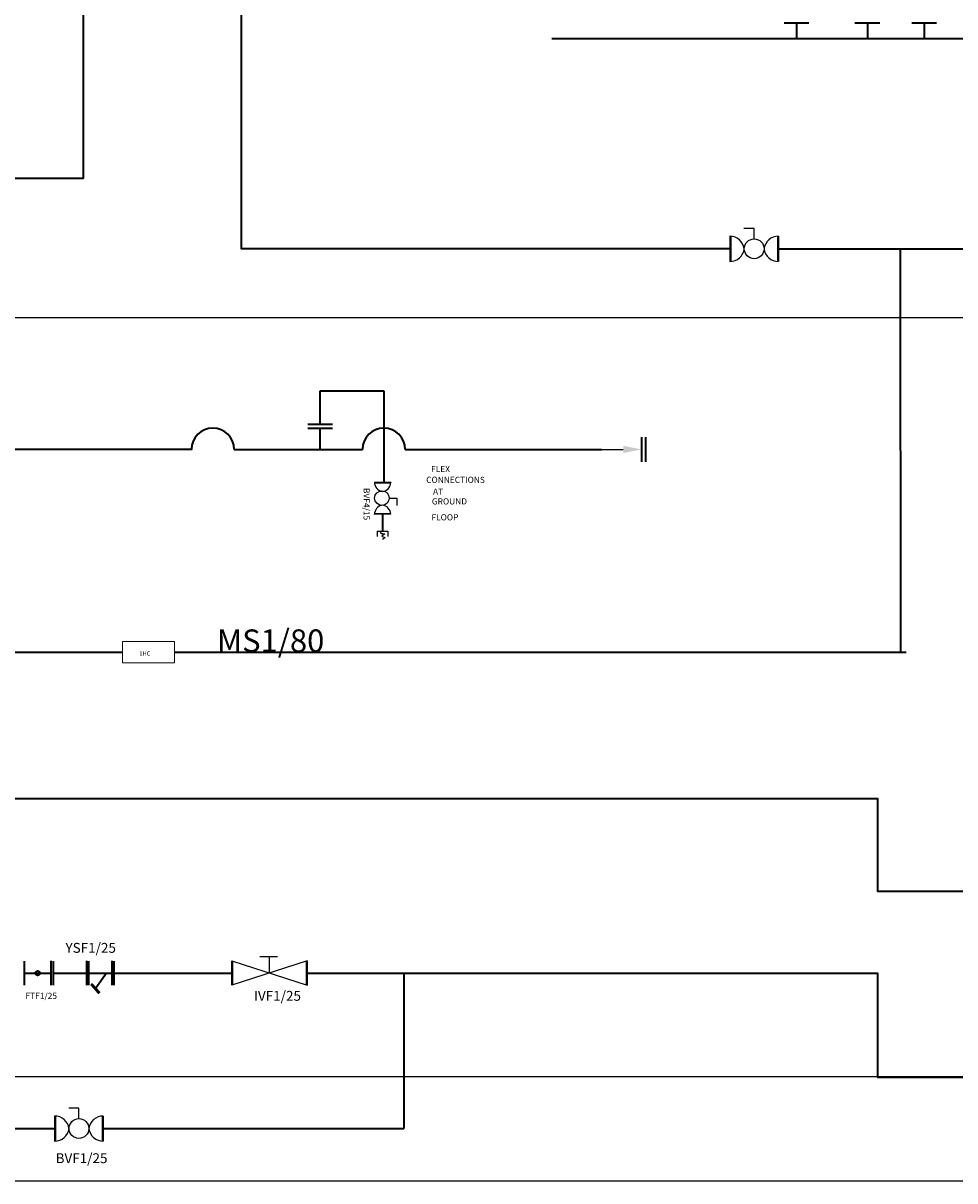
# Model space of a CAD drawing. Units: millimetres. Extents: x 353872 to 441597, y 126154 to 187356.
# Tile 6 of 28: x 381210 to 390443, y 137813 to 149281. Entities that reach past the tile are written whole.
import ezdxf

# ---------------------------------------------------------------- set-up
doc = ezdxf.new("R2010")
doc.units = ezdxf.units.MM
doc.linetypes.add('ACAD_ISO02W100', pattern=[15, 12, -3])
for name, color, linetype, lineweight in [('A-ANNO-DIMS', 2, 'Continuous', 18), ('P-ANNO-TEXT', 7, 'Continuous', 25), ('P-BNDY', 4, 'ACAD_ISO02W100', 25), ('P-INST', 6, 'Continuous', 25), ('P-INST-SIGN', 4, 'Continuous', 18), ('P-PIPE', 3, 'Continuous', 35), ('P-PIPE-FITT', 6, 'Continuous', 25), ('P-VALV', 2, 'Continuous', 25)]:
    doc.layers.add(name, color=color, linetype=linetype, lineweight=lineweight)
doc.layers.add('AC-UINT', color=2, linetype='Continuous')
doc.styles.get("Standard").update_dxf_attribs({"font": 'arial.ttf'})
doc.dimstyles.get("Standard").update_dxf_attribs({"dimtxt": 0.18, "dimasz": 0.18, "dimexe": 0.18, "dimexo": 0.0625, "dimgap": 0.09, "dimtad": 0, "dimtih": 1, "dimtoh": 1, "dimdec": 4, "dimzin": 0, "dimdsep": 46, "dimtxsty": 'Standard', "dimcen": 0.09, "dimadec": 0, "dimazin": 0, "dimtfac": 1, "dimtdec": 4, "dimtofl": 0, "dimtmove": 0, "dimatfit": 3, "dimfxl": 1, "dimtolj": 1, "dimtzin": 0, "dimarcsym": 0})

# ---------------------------------------------------------------- blocks, each defined once
blk = doc.blocks.new('DFSG')
at = {"layer": 'AC-UINT', "ltscale": 3}
blk.add_line((94.324, -27.16), (94.091, -27.16), dxfattribs=at)
blk.add_solid([(94.091, -27.121), (94.091, -27.199), (93.897, -27.16)], dxfattribs=at)
blk = doc.blocks.new('VALVE-A')
for points in [[(0, 9), (249, 9)], [(0, 6), (249, 6)], [(0, 3), (0, 0), (249, 0), (249, 4)], [(0, 3), (0, 3), (246, 3), (249, 3)]]:
    blk.add_lwpolyline(points)
for centre, radius, start, end in [((143, 1), 143, 97.3612, 180.5798), ((107, 2), 142, 359.2193, 82.8397)]:
    blk.add_arc(centre, radius, start, end)
blk = doc.blocks.new('VALVE-D-INDICATOR')
for points in [[(330, 249), (330, 0)], [(333, 249), (333, 0)], [(336, 249), (339, 249), (339, 0), (335, 0)], [(336, 249), (336, 246), (336, 3), (336, 0)]]:
    blk.add_lwpolyline(points)
blk.add_circle((98, 125), 98)
for centre, radius, start, end in [((338, 106), 143, 89.4202, 172.6388), ((337, 142), 142, 187.1603, 270.7807)]:
    blk.add_arc(centre, radius, start, end)
blk = doc.blocks.new('VALVE-K')
for points in [[(0, 91), (0, 93), (162, 93), (162, 90)], [(0, 91), (2, 91), (160, 91), (162, 91)], [(0, 89), (162, 89)], [(0, 87), (161, 87)]]:
    blk.add_lwpolyline(points)
for centre, radius, start, end in [((93, 92), 92.6, 179.4202, 262.6388), ((69, 92), 92.3, 277.1603, 0.7807)]:
    blk.add_arc(centre, radius, start, end)
blk = doc.blocks.new('INST-ELEMENT')
blk.add_lwpolyline([(145, 74), (220, 74), (220, 0)])
blk.add_circle((72, 74), 72.3)
blk = doc.blocks.new('*D27')
at = {"layer": 'A-ANNO-DIMS', "color": 0, "lineweight": -2, "transparency": 16777216}
for p, q in [((366977, 138848), (440591, 138848)), ((440591, 138848), (440591, 138331)), ((440591, 137813), (440591, 138330)), ((366977, 137813), (440591, 137813))]:
    blk.add_line(p, q, dxfattribs=at)
at = {"layer": 'A-ANNO-DIMS', "color": 0, "transparency": 16777216}
for points in [[(440591, 138848), (440591, 138848), (440591, 138848)], [(440591, 137813), (440591, 137813), (440591, 137813)]]:
    blk.add_solid(points, dxfattribs=at)
at = {"layer": 'Defpoints', "color": 0, "transparency": 16777216}
for p in [(366977, 138848), (366977, 137813), (440591, 137813)]:
    blk.add_point(p, dxfattribs=at)
at = {"layer": 'A-ANNO-DIMS', "color": 0, "transparency": 16777216, "insert": (440591, 138330), "char_height": 0.18, "attachment_point": 5}
blk.add_mtext('\\A1;1035.2', dxfattribs=at)

msp = doc.modelspace()

# ---------------------------------------------------------------- linework, layer by layer
at = {"layer": 'P-BNDY'}
msp.add_line((360736.55, 146365.61), (391507.08, 146365.61), dxfattribs=at)
at = {"layer": 'P-INST-SIGN'}
msp.add_lwpolyline([(382194.24, 143154.87), (382709.57, 143154.87), (382709.57, 142945.91), (382194.24, 142945.91)], close=True, dxfattribs=at)
at = {"layer": 'P-PIPE'}
for p, q in [((388996.7, 149280.57), (388751.94, 149280.57)), ((388874.32, 149280.57), (388874.32, 149129.17)), ((389698.22, 149280.57), (389453.46, 149280.57)), ((389575.84, 149280.57), (389575.84, 149129.17)), ((390262.67, 149280.57), (390017.91, 149280.57)), ((390140.29, 149280.57), (390140.29, 149129.17)), ((386450.69, 149129.17), (407087.67, 149129.17)), ((388692.41, 147045.54), (391112.65, 147045.74)), ((389902.53, 147045.64), (389902.86, 143050.39)), ((384154.35, 145309.55), (384154.35, 145637.47)), ((384154.35, 145637.47), (384783.69, 145637.47)), ((384783.69, 145637.47), (384783.69, 144732.81)), ((384031.97, 145309.55), (384276.73, 145309.55)), ((384031.97, 145270.39), (384276.73, 145270.39)), ((384154.35, 145058.64), (384154.35, 145270.39)), ((387336.62, 145179.44), (387336.62, 144934.68)), ((387375.77, 145179.44), (387375.77, 144934.68)), ((383301.45, 145058.64), (384571.94, 145058.64)), ((384995.44, 145058.64), (386942.19, 145058.64)), ((384771.93, 144414.6), (384771.93, 144247.55)), ((382709.57, 143050.39), (389961.77, 143050.39)), ((381219.87, 139989.74), (381219.87, 139751.19)), ((381485.14, 139991.02), (381485.14, 139752.47)), ((381505.55, 139989.74), (381505.55, 139751.19)), ((381838.28, 139991.02), (381838.28, 139752.47)), ((381858.69, 139989.74), (381858.69, 139751.19)), ((382088.51, 139991.02), (382088.51, 139752.47)), ((382108.93, 139989.74), (382108.93, 139751.19)), ((381219.87, 139870.46), (381485.14, 139870.46)), ((381505.55, 139870.46), (381838.28, 139870.46)), ((381858.69, 139870.46), (382088.51, 139870.46)), ((382035.97, 139870.46), (381929.73, 139721.6)), ((382108.93, 139870.46), (383279.44, 139870.46)), ((384981.21, 139870.46), (384981.21, 138330.46)), ((366976.76, 138330.45), (381521.27, 138330.45)), ((382003.25, 138330.46), (384981.21, 138330.46))]:
    msp.add_line(p, q, dxfattribs=at)
for points in [[(366976.76, 171744.89), (381803.29, 171744.89), (381803.29, 150820.94), (381803.29, 147742.48), (377889.79, 147742.48)], [(376740.39, 146769.18), (376740.39, 143050.39), (379096.81, 143050.39), (382194.24, 143050.39)], [(380161.54, 141602.11), (389676.87, 141602.11), (389676.87, 140682.39), (392361.87, 140682.39), (392361.87, 141110.07)], [(384023.46, 139870.46), (389676.87, 139870.46), (389676.87, 138839.25), (395834.15, 138839.25), (395834.15, 140770.36)]]:
    msp.add_lwpolyline(points, dxfattribs=at)
for points in [[(388213.21, 147045.52), (383375.2, 147045.17), (383375.2, 147045.17), (383375.2, 149602.24), (383375.2, 167832.6), (382147.59, 167832.6, 1), (381458.98, 167832.6), (380124.81, 167832.6, 1), (379436.2, 167832.6), (368453.37, 167832.6)], [(383301.45, 145058.64, 1), (382877.96, 145058.64), (377035.77, 145058.64, 1), (376445.02, 145058.64), (372504.41, 145058.64, 1), (371913.66, 145058.64), (366976.76, 145058.64)]]:
    msp.add_lwpolyline(points, format="xyb", dxfattribs=at)
msp.add_lwpolyline([(381884.53, 139753.44), (381894.08, 139761.89), (381965.38, 139681.3), (381955.83, 139672.85)], close=True, dxfattribs=at)
msp.add_circle((381353.34, 139870.46), 22.57, dxfattribs=at)
msp.add_arc((384783.69, 145058.64), 211.75, 0, 180, dxfattribs=at)
at = {"layer": 'P-VALV'}
for p, q in [((383555.44, 140034.39), (383731.66, 140034.39)), ((383651.45, 139870.46), (383651.45, 140034.39)), ((383279.44, 139991.02), (384023.46, 139749.91)), ((384023.46, 139991.02), (383279.44, 139749.91))]:
    msp.add_line(p, q, dxfattribs=at)
for points in [[(388454.2, 147143.89), (388454.2, 147246.54), (388353.42, 147246.54)], [(384720.39, 144195.79), (384720.39, 144247.55), (384823.46, 144247.55), (384823.46, 144195.79)], [(383279.44, 139749.91), (383279.44, 139991.02)], [(383287.34, 139752.47), (383287.34, 139988.45)], [(384015.55, 139988.45), (384015.55, 139752.47)], [(384023.46, 139991.02), (384023.46, 139749.91)], [(381762.26, 138428.82), (381762.26, 138531.46), (381661.48, 138531.46)]]:
    msp.add_lwpolyline(points, dxfattribs=at)
msp.add_open_spline([(384770.05, 144247.55), (384758.68, 144240.53), (384728.6, 144221.95), (384828.65, 144229.34), (384735.73, 144194.17), (384810.98, 144191.29), (384784.82, 144174.67), (384772.32, 144166.73)], degree=3, knots=[0, 0, 0, 0, 27.05142883, 71.59411322, 109.19990694, 141.17080136, 170.38673835, 170.38673835, 170.38673835, 170.38673835], dxfattribs=at)

# ---------------------------------------------------------------- block references
at = {"layer": 'P-INST'}
msp.add_blockref('INST-ELEMENT', (384692.53, 144501.83), dxfattribs=at)
at = {"layer": 'P-PIPE-FITT', "xscale": 923.3484342094463, "yscale": 923.3484342094463, "zscale": 923.3484342094463, "rotation": 179.9589088552121}
msp.add_blockref('DFSG', (474017.82, 119917.94), dxfattribs=at)
at = {"layer": 'P-VALV'}
for name, p, rotation in [('VALVE-A', (388213.21, 147169.91), 269.9999999999359), ('VALVE-K', (384691.22, 144641.64), 0.0028725521061233), ('VALVE-K', (384850.84, 144509.52), 181.3047895544739), ('VALVE-A', (381521.27, 138454.83), 269.9999999998651)]:
    msp.add_blockref(name, p, dxfattribs=dict(at, rotation=rotation))
for p in [(388356.18, 146921.16), (381664.23, 138206.08)]:
    msp.add_blockref('VALVE-D-INDICATOR', p, dxfattribs=at)

# ---------------------------------------------------------------- texts
at = {"layer": 'P-ANNO-TEXT'}
for s, height, p in [('FLEX', 60.86, (385252.41, 144833.81)), ('CONNECTIONS', 60.86, (385203.8, 144726.97)), ('AT', 60.86, (385271.85, 144610.43)), ('GROUND', 60.86, (385260.18, 144513.3)), ('FLOOP', 60.86, (385256.29, 144355.96)), ('MS1/80', 225.086, (383130.43, 143050.39)), ('1HC', 41.643, (382361.48, 143015.8)), ('YSF1/25', 98.09, (381629.31, 140071.86)), ('IVF1/25', 98.09, (383497.65, 139596.47)), ('FTF1/25', 60.86, (381232.99, 139615.22)), ('BVF1/25', 98.09, (381531.38, 137988.08))]:
    msp.add_text(s, height=height, dxfattribs=at).set_placement(p)
msp.add_text('BVF4/15', height=60.86, rotation=270, dxfattribs=at).set_placement((384583.15, 144676.57))

# ---------------------------------------------------------------- dimensions: what is measured, and where the dimension line sits
at = {"layer": 'A-ANNO-DIMS'}
dim = msp.add_linear_dim(base=(440591, 137812.84), p1=(366976.76, 138848.06), p2=(366976.76, 137812.84), angle=90, dimstyle='Standard', override={"dimdec": 1, "dimlfac": 1, "dimrnd": 0, "dimzin": 0, "dimdsep": 46, "dimlunit": 2}, dxfattribs=at)
dim.commit()
dim.dimension.update_dxf_attribs({"geometry": '*D27', "text_midpoint": (440591, 138330.45)})

doc.saveas('drawing.dxf')
